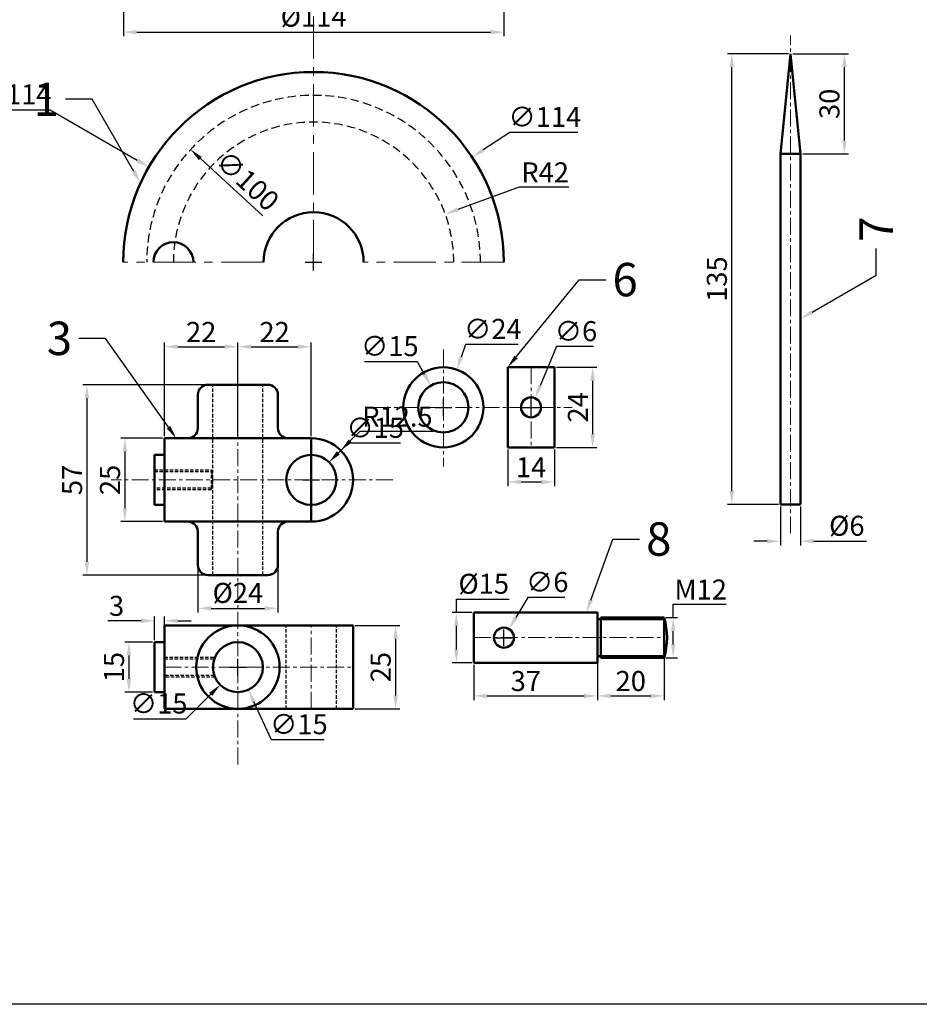
# Model space of a CAD drawing. Units: millimetres. Extents: x -65 to 576, y -103 to 374.
# Tile 2 of 4: x 81 to 351, y -103 to 192. Entities that reach past the tile are written whole.
import ezdxf
from ezdxf import colors
from ezdxf.entities.mleader import LeaderData, LeaderLine
from ezdxf.math import Vec2, Vec3

# ---------------------------------------------------------------- set-up
doc = ezdxf.new("R2010")
doc.units = ezdxf.units.MM
doc.header["$LTSCALE"] = 0.4
doc.linetypes.add('CENTER', pattern=[50.8, 31.75, -6.35, 6.35, -6.35])
doc.linetypes.add('HIDDEN', pattern=[9.525, 6.35, -3.175])
for name, color, linetype, lineweight in [('M-CNTR', 4, 'CENTER', 18), ('M-DIMS', 2, 'Continuous', 25), ('M-HIDN', 1, 'HIDDEN', 25), ('M-OUTL', 7, 'Continuous', 50), ('M-TEXT', 3, 'Continuous', 25), ('M-TTLB', 7, 'Continuous', 25)]:
    doc.layers.add(name, color=color, linetype=linetype, lineweight=lineweight)
doc.styles.get("Standard").update_dxf_attribs({"font": 'arial.ttf'})
doc.dimstyles.new('ISO-25', dxfattribs={"dimtxt": 6, "dimasz": 4, "dimexe": 1.25, "dimexo": 0.625, "dimtad": 1, "dimtoh": 1, "dimtxsty": 'Standard', "dimcen": 2.5, "dimadec": 0, "dimazin": 0, "dimtfac": 1, "dimtofl": 0, "dimtmove": 0, "dimatfit": 3, "dimfxl": 1, "dimarcsym": 0})

# ---------------------------------------------------------------- blocks, each defined once
blk = doc.blocks.new('*D1')
at = {"layer": 'Defpoints', "color": 0, "ltscale": 0.4, "transparency": 16777216}
for p in [(112.15, 220.83), (226.15, 220.83), (226.15, 187.9)]:
    blk.add_point(p, dxfattribs=at)
at = {"layer": 'M-DIMS', "color": 0, "lineweight": -2, "ltscale": 0.4, "transparency": 16777216}
for p, q in [((112.15, 220.2), (112.15, 186.65)), ((226.15, 220.2), (226.15, 186.65)), ((116.15, 187.9), (222.15, 187.9))]:
    blk.add_line(p, q, dxfattribs=at)
at = {"layer": 'M-DIMS', "color": 0, "ltscale": 0.4, "transparency": 16777216}
for points in [[(116.15, 188.57), (116.15, 187.24), (112.15, 187.9)], [(222.15, 188.57), (222.15, 187.24), (226.15, 187.9)]]:
    blk.add_solid(points, dxfattribs=at)
at = {"layer": 'M-DIMS', "color": 0, "ltscale": 0.4, "transparency": 16777216, "insert": (169.15, 191.76), "char_height": 6, "attachment_point": 5}
blk.add_mtext('%%C114', dxfattribs=at)
blk = doc.blocks.new('*D8')
at = {"layer": 'Defpoints', "color": 0, "ltscale": 0.4, "transparency": 16777216}
for p in [(216.68, 150.42), (121.61, 87.5)]:
    blk.add_point(p, dxfattribs=at)
at = {"layer": 'M-DIMS', "color": 0, "lineweight": -2, "ltscale": 0.4, "transparency": 16777216}
for p, q in [((227.95, 157.88), (220.01, 152.63)), ((248.33, 157.88), (227.95, 157.88)), ((169.15, 116.46), (169.15, 121.46)), ((166.65, 118.96), (171.65, 118.96))]:
    blk.add_line(p, q, dxfattribs=at)
at = {"layer": 'M-DIMS', "color": 0, "ltscale": 0.4, "transparency": 16777216}
blk.add_solid([(219.64, 153.18), (220.38, 152.07), (216.68, 150.42)], dxfattribs=at)
at = {"layer": 'M-DIMS', "color": 0, "ltscale": 0.4, "transparency": 16777216, "insert": (238.45, 161.73), "char_height": 6, "attachment_point": 5}
blk.add_mtext('∅114', dxfattribs=at)
blk = doc.blocks.new('*D9')
at = {"layer": 'Defpoints', "color": 0, "ltscale": 0.4, "transparency": 16777216}
for p in [(132.28, 152.73), (206.01, 85.18)]:
    blk.add_point(p, dxfattribs=at)
at = {"layer": 'M-DIMS', "color": 0, "lineweight": -2, "ltscale": 0.4, "transparency": 16777216}
blk.add_line((153.98, 132.85), (135.23, 150.03), dxfattribs=at)
at = {"layer": 'M-DIMS', "color": 0, "ltscale": 0.4, "transparency": 16777216}
blk.add_solid([(135.68, 150.52), (134.78, 149.54), (132.28, 152.73)], dxfattribs=at)
at = {"layer": 'M-DIMS', "color": 0, "ltscale": 0.4, "transparency": 16777216, "insert": (148.84, 142.79), "char_height": 6, "attachment_point": 5, "rotation": 317.5054}
blk.add_mtext('∅100', dxfattribs=at)
blk = doc.blocks.new('*D10')
at = {"layer": 'Defpoints', "color": 0, "ltscale": 0.4, "transparency": 16777216}
for p in [(208.59, 133.37), (169.15, 118.96)]:
    blk.add_point(p, dxfattribs=at)
at = {"layer": 'M-DIMS', "color": 0, "lineweight": -2, "ltscale": 0.4, "transparency": 16777216}
for p, q in [((230.77, 141.47), (212.35, 134.75)), ((245.67, 141.47), (230.77, 141.47)), ((169.15, 116.46), (169.15, 121.46)), ((166.65, 118.96), (171.65, 118.96))]:
    blk.add_line(p, q, dxfattribs=at)
at = {"layer": 'M-DIMS', "color": 0, "ltscale": 0.4, "transparency": 16777216}
blk.add_solid([(212.12, 135.37), (212.58, 134.12), (208.59, 133.37)], dxfattribs=at)
at = {"layer": 'M-DIMS', "color": 0, "ltscale": 0.4, "transparency": 16777216, "insert": (238.53, 145.11), "char_height": 6, "attachment_point": 5}
blk.add_mtext('R42', dxfattribs=at)
blk = doc.blocks.new('*D24')
at = {"layer": 'Defpoints', "color": 0, "ltscale": 0.4, "transparency": 16777216}
for p in [(312.08, 181.41), (328.19, 181.41), (315.08, 151.41)]:
    blk.add_point(p, dxfattribs=at)
at = {"layer": 'M-DIMS', "color": 0, "lineweight": -2, "ltscale": 0.4, "transparency": 16777216}
for p, q in [((312.71, 181.41), (329.44, 181.41)), ((328.19, 155.41), (328.19, 177.41)), ((315.71, 151.41), (329.44, 151.41))]:
    blk.add_line(p, q, dxfattribs=at)
at = {"layer": 'M-DIMS', "color": 0, "ltscale": 0.4, "transparency": 16777216}
for points in [[(327.53, 177.41), (328.86, 177.41), (328.19, 181.41)], [(327.53, 155.41), (328.86, 155.41), (328.19, 151.41)]]:
    blk.add_solid(points, dxfattribs=at)
at = {"layer": 'M-DIMS', "color": 0, "ltscale": 0.4, "transparency": 16777216, "insert": (324.5, 166.41), "char_height": 6, "attachment_point": 5, "rotation": 90}
blk.add_mtext('30', dxfattribs=at)
blk = doc.blocks.new('*D25')
at = {"layer": 'Defpoints', "color": 0, "ltscale": 0.4, "transparency": 16777216}
for p in [(294.46, 181.41), (312.08, 181.41), (309.08, 46.41)]:
    blk.add_point(p, dxfattribs=at)
at = {"layer": 'M-DIMS', "color": 0, "lineweight": -2, "ltscale": 0.4, "transparency": 16777216}
for p, q in [((311.46, 181.41), (293.21, 181.41)), ((294.46, 50.41), (294.46, 177.41)), ((308.46, 46.41), (293.21, 46.41))]:
    blk.add_line(p, q, dxfattribs=at)
at = {"layer": 'M-DIMS', "color": 0, "ltscale": 0.4, "transparency": 16777216}
for points in [[(293.79, 177.41), (295.13, 177.41), (294.46, 181.41)], [(293.79, 50.41), (295.13, 50.41), (294.46, 46.41)]]:
    blk.add_solid(points, dxfattribs=at)
at = {"layer": 'M-DIMS', "color": 0, "ltscale": 0.4, "transparency": 16777216, "insert": (290.77, 113.91), "char_height": 6, "attachment_point": 5, "rotation": 90}
blk.add_mtext('135', dxfattribs=at)
blk = doc.blocks.new('*D26')
at = {"layer": 'Defpoints', "color": 0, "ltscale": 0.4, "transparency": 16777216}
for p in [(309.08, 46.41), (315.08, 46.41), (315.08, 35.37)]:
    blk.add_point(p, dxfattribs=at)
at = {"layer": 'M-DIMS', "color": 0, "lineweight": -2, "ltscale": 0.4, "transparency": 16777216}
for p, q in [((309.08, 45.79), (309.08, 34.12)), ((315.08, 45.79), (315.08, 34.12)), ((305.08, 35.37), (301.08, 35.37)), ((319.08, 35.37), (334.79, 35.37))]:
    blk.add_line(p, q, dxfattribs=at)
at = {"layer": 'M-DIMS', "color": 0, "ltscale": 0.4, "transparency": 16777216}
for points in [[(305.08, 36.04), (305.08, 34.71), (309.08, 35.37)], [(319.08, 36.04), (319.08, 34.71), (315.08, 35.37)]]:
    blk.add_solid(points, dxfattribs=at)
at = {"layer": 'M-DIMS', "color": 0, "ltscale": 0.4, "transparency": 16777216, "insert": (328.93, 39.23), "char_height": 6, "attachment_point": 5}
blk.add_mtext('%%C6', dxfattribs=at)
blk = doc.blocks.new('*D27')
at = {"layer": 'Defpoints', "color": 0, "ltscale": 0.4, "transparency": 16777216}
for p in [(227.31, 63.48), (241.31, 63.48), (241.31, 53.14)]:
    blk.add_point(p, dxfattribs=at)
at = {"layer": 'M-DIMS', "color": 0, "lineweight": -2, "ltscale": 0.4, "transparency": 16777216}
for p, q in [((227.31, 62.86), (227.31, 51.89)), ((241.31, 62.86), (241.31, 51.89)), ((231.31, 53.14), (237.31, 53.14))]:
    blk.add_line(p, q, dxfattribs=at)
at = {"layer": 'M-DIMS', "color": 0, "ltscale": 0.4, "transparency": 16777216}
for points in [[(231.31, 53.81), (231.31, 52.48), (227.31, 53.14)], [(237.31, 53.81), (237.31, 52.48), (241.31, 53.14)]]:
    blk.add_solid(points, dxfattribs=at)
at = {"layer": 'M-DIMS', "color": 0, "ltscale": 0.4, "transparency": 16777216, "insert": (234.31, 56.78), "char_height": 6, "attachment_point": 5}
blk.add_mtext('14', dxfattribs=at)
blk = doc.blocks.new('*D28')
at = {"layer": 'Defpoints', "color": 0, "ltscale": 0.4, "transparency": 16777216}
for p in [(241.31, 87.48), (241.31, 63.48), (252.77, 63.48)]:
    blk.add_point(p, dxfattribs=at)
at = {"layer": 'M-DIMS', "color": 0, "lineweight": -2, "ltscale": 0.4, "transparency": 16777216}
for p, q in [((241.94, 87.48), (254.02, 87.48)), ((252.77, 83.48), (252.77, 67.48)), ((241.94, 63.48), (254.02, 63.48))]:
    blk.add_line(p, q, dxfattribs=at)
at = {"layer": 'M-DIMS', "color": 0, "ltscale": 0.4, "transparency": 16777216}
for points in [[(252.1, 83.48), (253.44, 83.48), (252.77, 87.48)], [(252.1, 67.48), (253.44, 67.48), (252.77, 63.48)]]:
    blk.add_solid(points, dxfattribs=at)
at = {"layer": 'M-DIMS', "color": 0, "ltscale": 0.4, "transparency": 16777216, "insert": (249.13, 75.48), "char_height": 6, "attachment_point": 5, "rotation": 90}
blk.add_mtext('24', dxfattribs=at)
blk = doc.blocks.new('*D29')
at = {"layer": 'Defpoints', "color": 0, "ltscale": 0.4, "transparency": 16777216}
for p in [(124.47, 66.24), (112.62, 41.24), (124.47, 41.24)]:
    blk.add_point(p, dxfattribs=at)
at = {"layer": 'M-DIMS', "color": 0, "lineweight": -2, "ltscale": 0.4, "transparency": 16777216}
for p, q in [((123.85, 66.24), (111.37, 66.24)), ((112.62, 62.24), (112.62, 45.24)), ((123.85, 41.24), (111.37, 41.24))]:
    blk.add_line(p, q, dxfattribs=at)
at = {"layer": 'M-DIMS', "color": 0, "ltscale": 0.4, "transparency": 16777216}
for points in [[(111.95, 62.24), (113.29, 62.24), (112.62, 66.24)], [(111.95, 45.24), (113.29, 45.24), (112.62, 41.24)]]:
    blk.add_solid(points, dxfattribs=at)
at = {"layer": 'M-DIMS', "color": 0, "ltscale": 0.4, "transparency": 16777216, "insert": (108.93, 53.74), "char_height": 6, "attachment_point": 5, "rotation": 90}
blk.add_mtext('25', dxfattribs=at)
blk = doc.blocks.new('*D30')
at = {"layer": 'Defpoints', "color": 0, "ltscale": 0.4, "transparency": 16777216}
for p in [(142.37, 82.24), (101.24, 25.24), (142.37, 25.24)]:
    blk.add_point(p, dxfattribs=at)
at = {"layer": 'M-DIMS', "color": 0, "lineweight": -2, "ltscale": 0.4, "transparency": 16777216}
for p, q in [((141.75, 82.24), (99.99, 82.24)), ((101.24, 78.24), (101.24, 29.24)), ((141.75, 25.24), (99.99, 25.24))]:
    blk.add_line(p, q, dxfattribs=at)
at = {"layer": 'M-DIMS', "color": 0, "ltscale": 0.4, "transparency": 16777216}
for points in [[(100.57, 78.24), (101.91, 78.24), (101.24, 82.24)], [(100.57, 29.24), (101.91, 29.24), (101.24, 25.24)]]:
    blk.add_solid(points, dxfattribs=at)
at = {"layer": 'M-DIMS', "color": 0, "ltscale": 0.4, "transparency": 16777216, "insert": (97.57, 53.74), "char_height": 6, "attachment_point": 5, "rotation": 90}
blk.add_mtext('57', dxfattribs=at)
blk = doc.blocks.new('*D31')
at = {"layer": 'Defpoints', "color": 0, "ltscale": 0.4, "transparency": 16777216}
for p in [(146.47, 93.65), (124.47, 66.24), (146.47, 66.24)]:
    blk.add_point(p, dxfattribs=at)
at = {"layer": 'M-DIMS', "color": 0, "lineweight": -2, "ltscale": 0.4, "transparency": 16777216}
for p, q in [((124.47, 66.87), (124.47, 94.9)), ((146.47, 66.87), (146.47, 94.9)), ((128.47, 93.65), (142.47, 93.65))]:
    blk.add_line(p, q, dxfattribs=at)
at = {"layer": 'M-DIMS', "color": 0, "ltscale": 0.4, "transparency": 16777216}
for points in [[(128.47, 94.32), (128.47, 92.99), (124.47, 93.65)], [(142.47, 94.32), (142.47, 92.99), (146.47, 93.65)]]:
    blk.add_solid(points, dxfattribs=at)
at = {"layer": 'M-DIMS', "color": 0, "ltscale": 0.4, "transparency": 16777216, "insert": (135.47, 97.29), "char_height": 6, "attachment_point": 5}
blk.add_mtext('22', dxfattribs=at)
blk = doc.blocks.new('*D32')
at = {"layer": 'Defpoints', "color": 0, "ltscale": 0.4, "transparency": 16777216}
for p in [(168.47, 93.65), (146.47, 66.24), (168.47, 66.24)]:
    blk.add_point(p, dxfattribs=at)
at = {"layer": 'M-DIMS', "color": 0, "lineweight": -2, "ltscale": 0.4, "transparency": 16777216}
for p, q in [((146.47, 66.87), (146.47, 94.9)), ((168.47, 66.87), (168.47, 94.9)), ((150.47, 93.65), (164.47, 93.65))]:
    blk.add_line(p, q, dxfattribs=at)
at = {"layer": 'M-DIMS', "color": 0, "ltscale": 0.4, "transparency": 16777216}
for points in [[(150.47, 94.32), (150.47, 92.99), (146.47, 93.65)], [(164.47, 94.32), (164.47, 92.99), (168.47, 93.65)]]:
    blk.add_solid(points, dxfattribs=at)
at = {"layer": 'M-DIMS', "color": 0, "ltscale": 0.4, "transparency": 16777216, "insert": (157.47, 97.29), "char_height": 6, "attachment_point": 5}
blk.add_mtext('22', dxfattribs=at)
blk = doc.blocks.new('*D33')
at = {"layer": 'Defpoints', "color": 0, "ltscale": 0.4, "transparency": 16777216}
for p in [(124.47, 11.55), (121.47, 5.16), (124.47, 5.16)]:
    blk.add_point(p, dxfattribs=at)
at = {"layer": 'M-DIMS', "color": 0, "lineweight": -2, "ltscale": 0.4, "transparency": 16777216}
for p, q in [((121.47, 5.78), (121.47, 12.8)), ((124.47, 5.78), (124.47, 12.8)), ((117.47, 11.55), (107.53, 11.55)), ((128.47, 11.55), (132.47, 11.55))]:
    blk.add_line(p, q, dxfattribs=at)
at = {"layer": 'M-DIMS', "color": 0, "ltscale": 0.4, "transparency": 16777216}
for points in [[(117.47, 12.21), (117.47, 10.88), (121.47, 11.55)], [(128.47, 12.21), (128.47, 10.88), (124.47, 11.55)]]:
    blk.add_solid(points, dxfattribs=at)
at = {"layer": 'M-DIMS', "color": 0, "ltscale": 0.4, "transparency": 16777216, "insert": (110.12, 15.24), "char_height": 6, "attachment_point": 5}
blk.add_mtext('3', dxfattribs=at)
blk = doc.blocks.new('*D34')
at = {"layer": 'Defpoints', "color": 0, "ltscale": 0.4, "transparency": 16777216}
for p in [(121.47, 5.16), (113.81, -9.84), (121.47, -9.84)]:
    blk.add_point(p, dxfattribs=at)
at = {"layer": 'M-DIMS', "color": 0, "lineweight": -2, "ltscale": 0.4, "transparency": 16777216}
for p, q in [((120.85, 5.16), (112.56, 5.16)), ((113.81, 1.16), (113.81, -5.84)), ((120.85, -9.84), (112.56, -9.84))]:
    blk.add_line(p, q, dxfattribs=at)
at = {"layer": 'M-DIMS', "color": 0, "ltscale": 0.4, "transparency": 16777216}
for points in [[(113.14, 1.16), (114.48, 1.16), (113.81, 5.16)], [(113.14, -5.84), (114.48, -5.84), (113.81, -9.84)]]:
    blk.add_solid(points, dxfattribs=at)
at = {"layer": 'M-DIMS', "color": 0, "ltscale": 0.4, "transparency": 16777216, "insert": (110.12, -2.34), "char_height": 6, "attachment_point": 5, "rotation": 90}
blk.add_mtext('15', dxfattribs=at)
blk = doc.blocks.new('*D35')
at = {"layer": 'Defpoints', "color": 0, "ltscale": 0.4, "transparency": 16777216}
for p in [(212.03, 86.8), (204.04, 64.17)]:
    blk.add_point(p, dxfattribs=at)
at = {"layer": 'M-DIMS', "color": 0, "lineweight": -2, "ltscale": 0.4, "transparency": 16777216}
for p, q in [((214.7, 94.34), (213.36, 90.57)), ((230.42, 94.34), (214.7, 94.34)), ((208.04, 72.98), (208.04, 77.98)), ((205.54, 75.48), (210.54, 75.48))]:
    blk.add_line(p, q, dxfattribs=at)
at = {"layer": 'M-DIMS', "color": 0, "ltscale": 0.4, "transparency": 16777216}
blk.add_solid([(212.74, 90.79), (213.99, 90.35), (212.03, 86.8)], dxfattribs=at)
at = {"layer": 'M-DIMS', "color": 0, "ltscale": 0.4, "transparency": 16777216, "insert": (222.87, 98.2), "char_height": 6, "attachment_point": 5}
blk.add_mtext('∅24', dxfattribs=at)
blk = doc.blocks.new('*D36')
at = {"layer": 'Defpoints', "color": 0, "ltscale": 0.4, "transparency": 16777216}
for p in [(204.31, 82), (211.76, 68.97)]:
    blk.add_point(p, dxfattribs=at)
at = {"layer": 'M-DIMS', "color": 0, "lineweight": -2, "ltscale": 0.4, "transparency": 16777216}
for p, q in [((184.41, 89.19), (200.2, 89.19)), ((200.2, 89.19), (202.33, 85.47)), ((208.04, 72.98), (208.04, 77.98)), ((205.54, 75.48), (210.54, 75.48))]:
    blk.add_line(p, q, dxfattribs=at)
at = {"layer": 'M-DIMS', "color": 0, "ltscale": 0.4, "transparency": 16777216}
blk.add_solid([(202.91, 85.8), (201.75, 85.14), (204.31, 82)], dxfattribs=at)
at = {"layer": 'M-DIMS', "color": 0, "ltscale": 0.4, "transparency": 16777216, "insert": (191.99, 93.05), "char_height": 6, "attachment_point": 5}
blk.add_mtext('∅15', dxfattribs=at)
blk = doc.blocks.new('*D37')
at = {"layer": 'Defpoints', "color": 0, "ltscale": 0.4, "transparency": 16777216}
for p in [(235.47, 78.25), (233.15, 72.72)]:
    blk.add_point(p, dxfattribs=at)
at = {"layer": 'M-DIMS', "color": 0, "lineweight": -2, "ltscale": 0.4, "transparency": 16777216}
for p, q in [((241.92, 93.68), (237.01, 81.94)), ((253, 93.68), (241.92, 93.68)), ((234.31, 72.98), (234.31, 77.98)), ((231.81, 75.48), (236.81, 75.48))]:
    blk.add_line(p, q, dxfattribs=at)
at = {"layer": 'M-DIMS', "color": 0, "ltscale": 0.4, "transparency": 16777216}
blk.add_solid([(236.4, 82.2), (237.63, 81.69), (235.47, 78.25)], dxfattribs=at)
at = {"layer": 'M-DIMS', "color": 0, "ltscale": 0.4, "transparency": 16777216, "insert": (247.78, 97.54), "char_height": 6, "attachment_point": 5}
blk.add_mtext('∅6', dxfattribs=at)
blk = doc.blocks.new('*D38')
at = {"layer": 'Defpoints', "color": 0, "ltscale": 0.4, "transparency": 16777216}
for p in [(180.97, 10.16), (180.97, -14.84), (193.72, -14.84)]:
    blk.add_point(p, dxfattribs=at)
at = {"layer": 'M-DIMS', "color": 0, "lineweight": -2, "ltscale": 0.4, "transparency": 16777216}
for p, q in [((181.6, 10.16), (194.97, 10.16)), ((193.72, 6.16), (193.72, -10.84)), ((181.6, -14.84), (194.97, -14.84))]:
    blk.add_line(p, q, dxfattribs=at)
at = {"layer": 'M-DIMS', "color": 0, "ltscale": 0.4, "transparency": 16777216}
for points in [[(193.06, 6.16), (194.39, 6.16), (193.72, 10.16)], [(193.06, -10.84), (194.39, -10.84), (193.72, -14.84)]]:
    blk.add_solid(points, dxfattribs=at)
at = {"layer": 'M-DIMS', "color": 0, "ltscale": 0.4, "transparency": 16777216, "insert": (190.04, -2.34), "char_height": 6, "attachment_point": 5, "rotation": 90}
blk.add_mtext('25', dxfattribs=at)
blk = doc.blocks.new('*D39')
at = {"layer": 'Defpoints', "color": 0, "ltscale": 0.4, "transparency": 16777216}
for p in [(143.32, 4.46), (149.62, -9.15)]:
    blk.add_point(p, dxfattribs=at)
at = {"layer": 'M-DIMS', "color": 0, "lineweight": -2, "ltscale": 0.4, "transparency": 16777216}
for p, q in [((146.47, -4.84), (146.47, 0.16)), ((143.97, -2.34), (148.97, -2.34)), ((156.54, -24.09), (151.3, -12.78)), ((172.33, -24.09), (156.54, -24.09))]:
    blk.add_line(p, q, dxfattribs=at)
at = {"layer": 'M-DIMS', "color": 0, "ltscale": 0.4, "transparency": 16777216}
blk.add_solid([(151.91, -12.5), (150.7, -13.06), (149.62, -9.15)], dxfattribs=at)
at = {"layer": 'M-DIMS', "color": 0, "ltscale": 0.4, "transparency": 16777216, "insert": (164.75, -20.24), "char_height": 6, "attachment_point": 5}
blk.add_mtext('∅15', dxfattribs=at)
blk = doc.blocks.new('*D40')
at = {"layer": 'Defpoints', "color": 0, "ltscale": 0.4, "transparency": 16777216}
for p in [(134.47, 33.24), (158.47, 33.24), (158.47, 15.27)]:
    blk.add_point(p, dxfattribs=at)
at = {"layer": 'M-DIMS', "color": 0, "lineweight": -2, "ltscale": 0.4, "transparency": 16777216}
for p, q in [((134.47, 32.62), (134.47, 14.02)), ((158.47, 32.62), (158.47, 14.02)), ((138.47, 15.27), (154.47, 15.27))]:
    blk.add_line(p, q, dxfattribs=at)
at = {"layer": 'M-DIMS', "color": 0, "ltscale": 0.4, "transparency": 16777216}
for points in [[(138.47, 15.93), (138.47, 14.6), (134.47, 15.27)], [(154.47, 15.93), (154.47, 14.6), (158.47, 15.27)]]:
    blk.add_solid(points, dxfattribs=at)
at = {"layer": 'M-DIMS', "color": 0, "ltscale": 0.4, "transparency": 16777216, "insert": (146.47, 19.12), "char_height": 6, "attachment_point": 5}
blk.add_mtext('%%C24', dxfattribs=at)
blk = doc.blocks.new('*D41')
at = {"layer": 'Defpoints', "color": 0, "ltscale": 0.4, "transparency": 16777216}
for p in [(217.19, 13.98), (211.93, -1.02), (217.19, -1.02)]:
    blk.add_point(p, dxfattribs=at)
at = {"layer": 'M-DIMS', "color": 0, "lineweight": -2, "ltscale": 0.4, "transparency": 16777216}
for p, q in [((211.93, 13.98), (211.93, 17.98)), ((211.93, 17.98), (227.72, 17.98)), ((216.57, 13.98), (210.68, 13.98)), ((211.93, 2.98), (211.93, 9.98)), ((216.57, -1.02), (210.68, -1.02))]:
    blk.add_line(p, q, dxfattribs=at)
at = {"layer": 'M-DIMS', "color": 0, "ltscale": 0.4, "transparency": 16777216}
for points in [[(211.27, 9.98), (212.6, 9.98), (211.93, 13.98)], [(211.27, 2.98), (212.6, 2.98), (211.93, -1.02)]]:
    blk.add_solid(points, dxfattribs=at)
at = {"layer": 'M-DIMS', "color": 0, "ltscale": 0.4, "transparency": 16777216, "insert": (220.14, 21.84), "char_height": 6, "attachment_point": 5}
blk.add_mtext('%%C15', dxfattribs=at)
blk = doc.blocks.new('*D42')
at = {"layer": 'Defpoints', "color": 0, "ltscale": 0.4, "transparency": 16777216}
for p in [(227.72, 9.07), (224.67, 3.9)]:
    blk.add_point(p, dxfattribs=at)
at = {"layer": 'M-DIMS', "color": 0, "lineweight": -2, "ltscale": 0.4, "transparency": 16777216}
for p, q in [((233.31, 18.54), (229.75, 12.51)), ((244.39, 18.54), (233.31, 18.54)), ((226.19, 3.98), (226.19, 8.98)), ((223.69, 6.48), (228.69, 6.48))]:
    blk.add_line(p, q, dxfattribs=at)
at = {"layer": 'M-DIMS', "color": 0, "ltscale": 0.4, "transparency": 16777216}
blk.add_solid([(229.18, 12.85), (230.33, 12.17), (227.72, 9.07)], dxfattribs=at)
at = {"layer": 'M-DIMS', "color": 0, "ltscale": 0.4, "transparency": 16777216, "insert": (239.16, 22.39), "char_height": 6, "attachment_point": 5}
blk.add_mtext('∅6', dxfattribs=at)
blk = doc.blocks.new('*D43')
at = {"layer": 'Defpoints', "color": 0, "ltscale": 0.4, "transparency": 16777216}
for p in [(217.19, -1.02), (254.19, -1.02), (254.19, -10.97)]:
    blk.add_point(p, dxfattribs=at)
at = {"layer": 'M-DIMS', "color": 0, "lineweight": -2, "ltscale": 0.4, "transparency": 16777216}
for p, q in [((217.19, -1.64), (217.19, -12.22)), ((254.19, -1.64), (254.19, -12.22)), ((221.19, -10.97), (250.19, -10.97))]:
    blk.add_line(p, q, dxfattribs=at)
at = {"layer": 'M-DIMS', "color": 0, "ltscale": 0.4, "transparency": 16777216}
for points in [[(221.19, -10.31), (221.19, -11.64), (217.19, -10.97)], [(250.19, -10.31), (250.19, -11.64), (254.19, -10.97)]]:
    blk.add_solid(points, dxfattribs=at)
at = {"layer": 'M-DIMS', "color": 0, "ltscale": 0.4, "transparency": 16777216, "insert": (232.75, -7.28), "char_height": 6, "attachment_point": 5}
blk.add_mtext('37', dxfattribs=at)
blk = doc.blocks.new('*D44')
at = {"layer": 'Defpoints', "color": 0, "ltscale": 0.4, "transparency": 16777216}
for p in [(254.19, 6.48), (274.19, 6.48), (274.19, -10.97)]:
    blk.add_point(p, dxfattribs=at)
at = {"layer": 'M-DIMS', "color": 0, "lineweight": -2, "ltscale": 0.4, "transparency": 16777216}
for p, q in [((254.19, 5.86), (254.19, -12.22)), ((274.19, 5.86), (274.19, -12.22)), ((258.19, -10.97), (270.19, -10.97))]:
    blk.add_line(p, q, dxfattribs=at)
at = {"layer": 'M-DIMS', "color": 0, "ltscale": 0.4, "transparency": 16777216}
for points in [[(258.19, -10.31), (258.19, -11.64), (254.19, -10.97)], [(270.19, -10.31), (270.19, -11.64), (274.19, -10.97)]]:
    blk.add_solid(points, dxfattribs=at)
at = {"layer": 'M-DIMS', "color": 0, "ltscale": 0.4, "transparency": 16777216, "insert": (264.19, -7.28), "char_height": 6, "attachment_point": 5}
blk.add_mtext('20', dxfattribs=at)
blk = doc.blocks.new('*D45')
at = {"layer": 'Defpoints', "color": 0, "ltscale": 0.4, "transparency": 16777216}
for p in [(274.19, 12.48), (274.19, 0.48), (276.9, 0.48)]:
    blk.add_point(p, dxfattribs=at)
at = {"layer": 'M-DIMS', "color": 0, "lineweight": -2, "ltscale": 0.4, "transparency": 16777216}
for p, q in [((276.9, 12.48), (276.9, 16.48)), ((276.9, 16.48), (292.76, 16.48)), ((274.82, 12.48), (278.15, 12.48)), ((276.9, 4.48), (276.9, 8.48)), ((274.82, 0.48), (278.15, 0.48))]:
    blk.add_line(p, q, dxfattribs=at)
at = {"layer": 'M-DIMS', "color": 0, "ltscale": 0.4, "transparency": 16777216}
for points in [[(276.23, 8.48), (277.56, 8.48), (276.9, 12.48)], [(276.23, 4.48), (277.56, 4.48), (276.9, 0.48)]]:
    blk.add_solid(points, dxfattribs=at)
at = {"layer": 'M-DIMS', "color": 0, "ltscale": 0.4, "transparency": 16777216, "insert": (285.14, 20.12), "char_height": 6, "attachment_point": 5}
blk.add_mtext('M12', dxfattribs=at)
blk = doc.blocks.new('*D56')
at = {"layer": 'Defpoints', "color": 0, "ltscale": 0.4, "transparency": 16777216}
for p in [(119.8, 147.5), (218.49, 90.42)]:
    blk.add_point(p, dxfattribs=at)
at = {"layer": 'M-DIMS', "color": 0, "lineweight": -2, "ltscale": 0.4, "transparency": 16777216}
for p, q in [((69.82, 164.62), (90.2, 164.62)), ((90.2, 164.62), (116.34, 149.5)), ((169.15, 116.46), (169.15, 121.46)), ((166.65, 118.96), (171.65, 118.96))]:
    blk.add_line(p, q, dxfattribs=at)
at = {"layer": 'M-DIMS', "color": 0, "ltscale": 0.4, "transparency": 16777216}
blk.add_solid([(116.68, 150.08), (116.01, 148.92), (119.8, 147.5)], dxfattribs=at)
at = {"layer": 'M-DIMS', "color": 0, "ltscale": 0.4, "transparency": 16777216, "insert": (79.7, 168.48), "char_height": 6, "attachment_point": 5}
blk.add_mtext('∅114', dxfattribs=at)
blk = doc.blocks.new('*D57')
at = {"layer": 'Defpoints', "color": 0, "ltscale": 0.4, "transparency": 16777216}
for p in [(173.77, 59.05), (163.17, 48.44)]:
    blk.add_point(p, dxfattribs=at)
at = {"layer": 'M-DIMS', "color": 0, "lineweight": -2, "ltscale": 0.4, "transparency": 16777216}
for p, q in [((179.42, 64.71), (176.6, 61.88)), ((195.22, 64.71), (179.42, 64.71)), ((168.47, 51.24), (168.47, 56.24)), ((165.97, 53.74), (170.97, 53.74))]:
    blk.add_line(p, q, dxfattribs=at)
at = {"layer": 'M-DIMS', "color": 0, "ltscale": 0.4, "transparency": 16777216}
blk.add_solid([(176.13, 62.35), (177.07, 61.41), (173.77, 59.05)], dxfattribs=at)
at = {"layer": 'M-DIMS', "color": 0, "ltscale": 0.4, "transparency": 16777216, "insert": (187.63, 68.57), "char_height": 6, "attachment_point": 5}
blk.add_mtext('∅15', dxfattribs=at)
blk = doc.blocks.new('*D58')
at = {"layer": 'Defpoints', "color": 0, "ltscale": 0.4, "transparency": 16777216}
for p in [(177.31, 62.58), (168.47, 53.74)]:
    blk.add_point(p, dxfattribs=at)
at = {"layer": 'M-DIMS', "color": 0, "lineweight": -2, "ltscale": 0.4, "transparency": 16777216}
for p, q in [((182.97, 68.24), (180.14, 65.41)), ((204.97, 68.24), (182.97, 68.24)), ((168.47, 51.24), (168.47, 56.24)), ((165.97, 53.74), (170.97, 53.74))]:
    blk.add_line(p, q, dxfattribs=at)
at = {"layer": 'M-DIMS', "color": 0, "ltscale": 0.4, "transparency": 16777216}
blk.add_solid([(179.67, 65.88), (180.61, 64.94), (177.31, 62.58)], dxfattribs=at)
at = {"layer": 'M-DIMS', "color": 0, "ltscale": 0.4, "transparency": 16777216, "insert": (194.28, 71.93), "char_height": 6, "attachment_point": 5}
blk.add_mtext('R12.5', dxfattribs=at)
blk = doc.blocks.new('*D59')
at = {"layer": 'Defpoints', "color": 0, "ltscale": 0.4, "transparency": 16777216}
for p in [(151.77, 2.96), (141.17, -7.65)]:
    blk.add_point(p, dxfattribs=at)
at = {"layer": 'M-DIMS', "color": 0, "lineweight": -2, "ltscale": 0.4, "transparency": 16777216}
for p, q in [((146.47, -4.84), (146.47, 0.16)), ((143.97, -2.34), (148.97, -2.34)), ((130.95, -17.88), (138.34, -10.48)), ((115.15, -17.88), (130.95, -17.88))]:
    blk.add_line(p, q, dxfattribs=at)
at = {"layer": 'M-DIMS', "color": 0, "ltscale": 0.4, "transparency": 16777216}
blk.add_solid([(137.87, -10.01), (138.81, -10.95), (141.17, -7.65)], dxfattribs=at)
at = {"layer": 'M-DIMS', "color": 0, "ltscale": 0.4, "transparency": 16777216, "insert": (122.74, -14.02), "char_height": 6, "attachment_point": 5}
blk.add_mtext('∅15', dxfattribs=at)

msp = doc.modelspace()

# ---------------------------------------------------------------- linework, layer by layer
at = {"layer": 'M-CNTR'}
for p, q in [((169.146, 118.958), (169.146, 248.195)), ((154.146, 118.958), (112.146, 118.958)), ((226.146, 118.958), (184.146, 118.958))]:
    msp.add_line(p, q, dxfattribs=at)
at = {"layer": 'M-CNTR', "ltscale": 0.4}
for p, q in [((312.081, 37.744), (312.081, 186.935)), ((208.038, 92.848), (208.038, 57.733)), ((234.311, 87.485), (234.311, 63.485)), ((146.472, -31.53), (146.472, 82.245)), ((187.247, 75.485), (246.603, 75.485)), ((192.89, 53.745), (108.531, 53.745)), ((168.472, -14.845), (168.472, 10.155)), ((217.192, 6.484), (274.192, 6.484)), ((124.472, -2.345), (180.972, -2.345))]:
    msp.add_line(p, q, dxfattribs=at)
at = {"layer": 'M-HIDN', "ltscale": 0.4}
for p, q in [((138.972, 25.245), (138.972, 82.245)), ((153.972, 25.245), (153.972, 82.245)), ((121.472, 56.745), (138.472, 56.745)), ((121.472, 56.245), (138.472, 56.245)), ((138.472, 56.745), (138.472, 50.745)), ((138.472, 51.245), (121.472, 51.245)), ((138.472, 50.745), (121.472, 50.745)), ((160.972, -14.845), (160.972, 10.155)), ((175.972, -14.845), (175.972, 10.155)), ((124.472, 0.655), (139.598, 0.655)), ((124.472, 0.155), (139.401, 0.155)), ((139.401, -4.845), (124.472, -4.845)), ((139.598, -5.345), (124.472, -5.345))]:
    msp.add_line(p, q, dxfattribs=at)
at = {"layer": 'M-HIDN'}
for radius in [50, 42]:
    msp.add_arc((169.146, 118.958), radius, 0, 180, dxfattribs=at)
at = {"layer": 'M-HIDN', "ltscale": 0.4}
msp.add_arc((128.842, 53.745), 10.086, 342.69568, 17.30432, dxfattribs=at)
at = {"layer": 'M-OUTL', "ltscale": 0.4}
for p, q in [((309.081, 151.411), (312.081, 181.411)), ((312.081, 181.411), (315.081, 151.411)), ((309.081, 46.411), (309.081, 151.411)), ((309.081, 151.411), (315.081, 151.411)), ((315.081, 151.411), (315.081, 46.411)), ((227.311, 87.485), (227.311, 63.485)), ((241.311, 87.485), (227.311, 87.485)), ((241.311, 63.485), (241.311, 87.485)), ((155.472, 82.245), (137.472, 82.245)), ((134.472, 69.245), (134.472, 79.245)), ((158.472, 69.245), (158.472, 79.245)), ((124.472, 41.245), (124.472, 66.245)), ((124.472, 66.245), (131.472, 66.245)), ((131.472, 66.245), (161.472, 66.245)), ((161.472, 66.245), (168.472, 66.245)), ((168.472, 41.245), (168.472, 66.245)), ((227.311, 63.485), (241.311, 63.485)), ((124.472, 61.245), (121.472, 61.245)), ((121.472, 61.245), (121.472, 46.245)), ((121.472, 46.245), (124.472, 46.245)), ((315.081, 46.411), (309.081, 46.411)), ((131.472, 41.245), (124.472, 41.245)), ((161.472, 41.245), (131.472, 41.245)), ((168.472, 41.245), (161.472, 41.245)), ((134.472, 28.245), (134.472, 38.245)), ((158.472, 28.245), (158.472, 38.245)), ((155.472, 25.245), (137.472, 25.245)), ((217.192, 13.984), (217.192, -1.016)), ((254.192, 13.984), (217.192, 13.984)), ((254.192, -1.016), (254.192, 13.984)), ((254.192, 11.984), (274.192, 11.984)), ((255.192, 12.484), (274.192, 12.484)), ((255.192, 0.484), (255.192, 12.484)), ((274.192, 12.484), (274.192, 0.484)), ((124.472, -14.845), (124.472, 10.155)), ((124.472, 10.155), (131.472, 10.155)), ((131.472, 10.155), (180.972, 10.155)), ((161.472, 10.155), (168.472, 10.155)), ((180.972, -14.845), (180.972, 10.155)), ((124.472, 5.155), (121.472, 5.155)), ((121.472, 5.155), (121.472, -9.845)), ((274.192, 0.984), (254.192, 0.984)), ((274.192, 0.484), (255.192, 0.484)), ((217.192, -1.016), (254.192, -1.016)), ((121.472, -9.845), (124.472, -9.845)), ((131.472, -14.845), (124.472, -14.845)), ((180.972, -14.845), (131.472, -14.845)), ((168.472, -14.845), (161.472, -14.845))]:
    msp.add_line(p, q, dxfattribs=at)
for centre, radius in [((208.038, 75.485), 12), ((208.038, 75.485), 7.5), ((234.311, 75.485), 3), ((168.472, 53.745), 7.5), ((146.472, -2.345), 12.5), ((226.192, 6.484), 3), ((146.472, -2.345), 7.5)]:
    msp.add_circle(centre, radius, dxfattribs=at)
at = {"layer": 'M-OUTL'}
for radius in [57, 15]:
    msp.add_arc((169.146, 118.958), radius, 0, 180, dxfattribs=at)
at = {"layer": 'M-OUTL', "ltscale": 0.4}
for centre, radius, start, end in [((127.146, 118.958), 6, 0, 180), ((137.472, 79.245), 3, 90, 180), ((155.472, 79.245), 3, 0, 90), ((131.472, 69.245), 3, 270, 0), ((161.472, 69.245), 3, 180, 270), ((168.472, 53.745), 12.5, 270, 90), ((131.472, 38.245), 3, 0, 90), ((161.472, 38.245), 3, 90, 180), ((137.472, 28.245), 3, 180, 270), ((155.472, 28.245), 3, 270, 0), ((253.736, 6.484), 21.318, 343.65297, 16.34703)]:
    msp.add_arc(centre, radius, start, end, dxfattribs=at)
at = {"layer": 'M-TTLB', "ltscale": 0.4}
msp.add_lwpolyline([(-64.629, 373.834), (576.345, 373.834), (576.345, -103.363), (-64.629, -103.363)], close=True, dxfattribs=at)

# ---------------------------------------------------------------- dimensions: what is measured, and where the dimension line sits
at = {"layer": 'M-DIMS', "ltscale": 0.4}
dim = msp.add_linear_dim(base=(226.146, 187.903), p1=(112.146, 220.828), p2=(226.146, 220.828), text='%%C<>', dimstyle='ISO-25', override={"dimclrd": 0, "dimclre": 0, "dimclrt": 0}, dxfattribs=at)
dim.commit()
dim.dimension.update_dxf_attribs({"geometry": '*D1', "text_midpoint": (169.146, 187.903), "dimtype": 160})
for base, p1, p2, picture, middle in [((294.459, 181.411), (309.081, 46.411), (312.081, 181.411), '*D25', (290.768, 113.911)), ((328.192, 181.411), (315.081, 151.411), (312.081, 181.411), '*D24', (324.502, 166.411)), ((252.769, 63.485), (241.311, 87.485), (241.311, 63.485), '*D28', (249.132, 75.485)), ((101.241, 25.245), (142.374, 82.245), (142.374, 25.245), '*D30', (97.565, 53.745)), ((112.621, 41.245), (124.472, 66.245), (124.472, 41.245), '*D29', (108.933, 53.745)), ((193.723, -14.845), (180.972, 10.155), (180.972, -14.845), '*D38', (190.035, -2.345)), ((113.81, -9.845), (121.472, 5.155), (121.472, -9.845), '*D34', (110.121, -2.345))]:
    dim = msp.add_linear_dim(base=base, p1=p1, p2=p2, angle=90, dimstyle='ISO-25', override={"dimclrd": 0, "dimclre": 0, "dimclrt": 0}, dxfattribs=at)
    dim.commit()
    dim.dimension.update_dxf_attribs({"geometry": picture, "text_midpoint": middle})
for p1, p2, override, picture, middle in [((218.486, 90.418), (119.805, 147.497), {"dimdec": 0, "dimlfac": 1, "dimrnd": 0, "dimzin": 0, "dimdsep": 46, "dimlunit": 2}, '*D56', (79.696, 164.621)), ((121.614, 87.497), (216.677, 150.418), {"dimclrd": 0, "dimclre": 0, "dimclrt": 0}, '*D8', (238.453, 157.878)), ((206.013, 85.182), (132.279, 152.734), {"dimclrd": 0, "dimclre": 0, "dimclrt": 0}, '*D9', (146.233, 139.949)), ((233.154, 72.717), (235.468, 78.252), {"dimclrd": 0, "dimclre": 0, "dimclrt": 0}, '*D37', (247.775, 93.685)), ((211.761, 68.974), (204.314, 81.995), {"dimclrd": 0, "dimclre": 0, "dimclrt": 0}, '*D36', (191.99, 89.192)), ((163.172, 48.438), (173.771, 59.051), {"dimdec": 0, "dimlfac": 1, "dimrnd": 0, "dimzin": 0, "dimdsep": 46, "dimlunit": 2}, '*D57', (187.633, 64.712)), ((224.667, 3.901), (227.718, 9.067), {"dimclrd": 0, "dimclre": 0, "dimclrt": 0}, '*D42', (239.165, 18.535)), ((151.773, 2.96), (141.17, -7.65), {"dimdec": 0, "dimlfac": 1, "dimrnd": 0, "dimzin": 0, "dimdsep": 46, "dimlunit": 2}, '*D59', (122.738, -17.88)), ((143.32, 4.461), (149.623, -9.151), {"dimclrd": 0, "dimclre": 0, "dimclrt": 0}, '*D39', (164.751, -24.094))]:
    dim = msp.add_diameter_dim_2p(p1=p1, p2=p2, dimstyle='ISO-25', override=override, dxfattribs=at)
    dim.commit()
    dim.dimension.update_dxf_attribs({"geometry": picture, "text_midpoint": middle, "dimtype": 163})
dim = msp.add_radius_dim(center=(169.146, 118.958), mpoint=(208.594, 133.373), dimstyle='ISO-25', override={"dimclrd": 0, "dimclre": 0, "dimclrt": 0}, dxfattribs=at)
dim.commit()
dim.dimension.update_dxf_attribs({"geometry": '*D10', "text_midpoint": (238.528, 141.474), "dimtype": 164})
for base, p1, p2, picture, middle in [((146.472, 93.653), (124.472, 66.245), (146.472, 66.245), '*D31', (135.472, 97.29)), ((168.472, 93.653), (146.472, 66.245), (168.472, 66.245), '*D32', (157.472, 97.29)), ((241.311, 53.142), (227.311, 63.485), (241.311, 63.485), '*D27', (234.311, 56.779)), ((274.192, -10.972), (254.192, 6.484), (274.192, 6.484), '*D44', (264.192, -7.284))]:
    dim = msp.add_linear_dim(base=base, p1=p1, p2=p2, dimstyle='ISO-25', override={"dimclrd": 0, "dimclre": 0, "dimclrt": 0}, dxfattribs=at)
    dim.commit()
    dim.dimension.update_dxf_attribs({"geometry": picture, "text_midpoint": middle})
dim = msp.add_diameter_dim_2p(p1=(204.043, 64.169), p2=(212.033, 86.8), dimstyle='ISO-25', override={"dimclrd": 0, "dimclre": 0, "dimclrt": 0}, dxfattribs=at)
dim.commit()
dim.dimension.update_dxf_attribs({"geometry": '*D35', "text_midpoint": (222.87, 98.2)})
dim = msp.add_radius_dim(center=(168.472, 53.745), mpoint=(177.312, 62.582), dimstyle='ISO-25', override={"dimdec": 1, "dimlfac": 1, "dimrnd": 0, "dimzin": 0, "dimdsep": 46, "dimlunit": 2}, dxfattribs=at)
dim.commit()
dim.dimension.update_dxf_attribs({"geometry": '*D58', "text_midpoint": (194.281, 71.926)})
dim = msp.add_linear_dim(base=(315.081, 35.373), p1=(309.081, 46.411), p2=(315.081, 46.411), angle=180, text='%%C<>', dimstyle='ISO-25', override={"dimclrd": 0, "dimclre": 0, "dimclrt": 0}, dxfattribs=at)
dim.commit()
dim.dimension.update_dxf_attribs({"geometry": '*D26', "text_midpoint": (328.934, 39.23)})
dim = msp.add_linear_dim(base=(158.472, 15.268), p1=(134.472, 33.245), p2=(158.472, 33.245), text='%%C<>', dimstyle='ISO-25', override={"dimclrd": 0, "dimclre": 0, "dimclrt": 0}, dxfattribs=at)
dim.commit()
dim.dimension.update_dxf_attribs({"geometry": '*D40', "text_midpoint": (146.472, 19.124)})
for base, p1, p2, text, picture, middle in [((211.932, -1.016), (217.192, 13.984), (217.192, -1.016), '%%C<>', '*D41', (220.141, 17.984)), ((276.897, 0.484), (274.192, 12.484), (274.192, 0.484), 'M<>', '*D45', (285.143, 16.484))]:
    dim = msp.add_linear_dim(base=base, p1=p1, p2=p2, angle=90, text=text, dimstyle='ISO-25', override={"dimclrd": 0, "dimclre": 0, "dimclrt": 0}, dxfattribs=at)
    dim.commit()
    dim.dimension.update_dxf_attribs({"geometry": picture, "text_midpoint": middle, "dimtype": 160})
for base, p1, p2, picture, middle in [((124.472, 11.546), (121.472, 5.155), (124.472, 5.155), '*D33', (110.123, 11.546)), ((254.192, -10.972), (217.192, -1.016), (254.192, -1.016), '*D43', (232.747, -10.972))]:
    dim = msp.add_linear_dim(base=base, p1=p1, p2=p2, dimstyle='ISO-25', override={"dimclrd": 0, "dimclre": 0, "dimclrt": 0}, dxfattribs=at)
    dim.commit()
    dim.dimension.update_dxf_attribs({"geometry": picture, "text_midpoint": middle, "dimtype": 160})

# ---------------------------------------------------------------- leaders
at = {"layer": 'M-TEXT', "ltscale": 0.4}
ml = msp.add_multileader_mtext('Standard', dxfattribs=at)
ml.set_content('1', color=256)
ml.set_leader_properties()
ml.build(insert=Vec2(0, 0))
ctx = ml.context
ctx.base_point, ctx.char_height, ctx.plane_origin = Vec3(87.133, 167.794), 10, Vec3(117.316, 142.679)
ctx.text_align_type = 2
notes = []
notes.append((ctx, [(0, (1, 1, 0), (102.816, 167.794), (-1, 0), 8, [(0, [(117.316, 142.679)], 0, [])])]))
ctx.mtext.insert, ctx.mtext.alignment, ctx.mtext.flow_direction = Vec3(92.816, 172.794), 3, 5
ml = msp.add_multileader_mtext('Standard', dxfattribs=at)
ml.set_content('7', color=256)
ml.set_leader_properties()
ml.build(insert=Vec2(0, 0))
ctx = ml.context
ctx.base_point, ctx.char_height, ctx.plane_origin, ctx.plane_x_axis, ctx.plane_y_axis = Vec3(337.727, 123.094), 10, Vec3(315.081, 102.019), Vec3(0, 1), Vec3(-1, 0)
notes.append((ctx, [(0, (1, 1, 0), (337.727, 115.094), (0, 1), 8, [(0, [(315.081, 102.019)], 0, [])])]))
ctx.mtext.insert, ctx.mtext.text_direction, ctx.mtext.rotation, ctx.mtext.flow_direction = Vec3(332.727, 125.094), Vec3(0, 1), 1.5707963, 5
ml = msp.add_multileader_mtext('Standard', dxfattribs=at)
ml.set_content('6', color=256)
ml.set_leader_properties()
ml.build(insert=Vec2(0, 0))
ctx = ml.context
ctx.base_point, ctx.char_height, ctx.plane_origin = Vec3(256.712, 113.672), 10, Vec3(227.311, 87.485)
notes.append((ctx, [(0, (1, 1, 0), (248.712, 113.672), (1, 0), 8, [(0, [(227.311, 87.485)], 0, [])])]))
ctx.mtext.insert, ctx.mtext.flow_direction = Vec3(258.712, 118.757), 5
ml = msp.add_multileader_mtext('Standard', dxfattribs=at)
ml.set_content('3', color=256)
ml.set_leader_properties()
ml.build(insert=Vec2(0, 0))
ctx = ml.context
ctx.base_point, ctx.char_height, ctx.plane_origin = Vec3(88.231, 96.074), 10, Vec3(127.972, 66.245)
ctx.text_align_type = 2
notes.append((ctx, [(0, (1, 1, 0), (106.779, 96.074), (-1, 0), 8, [(0, [(127.972, 66.245)], 0, [])])]))
ctx.mtext.insert, ctx.mtext.alignment, ctx.mtext.flow_direction = Vec3(96.779, 101.163), 3, 5
ml = msp.add_multileader_mtext('Standard', dxfattribs=at)
ml.set_content('8', color=256)
ml.set_leader_properties()
ml.build(insert=Vec2(0, 0))
ctx = ml.context
ctx.base_point, ctx.char_height, ctx.plane_origin = Vec3(266.8, 35.955), 10, Vec3(250.86, 13.984)
notes.append((ctx, [(0, (1, 1, 0), (258.8, 35.955), (1, 0), 8, [(0, [(250.86, 13.984)], 0, [])])]))
ctx.mtext.insert, ctx.mtext.flow_direction = Vec3(268.8, 41.04), 5
for ctx, leaders in notes:
    for number, flags, end, landing, length, lines in leaders:
        leader = LeaderData()
        leader.index, (leader.has_last_leader_line, leader.has_dogleg_vector, leader.attachment_direction) = number, flags
        leader.last_leader_point, leader.dogleg_vector, leader.dogleg_length = Vec3(end), Vec3(landing), length
        for number, points, colour, breaks in lines:
            line = LeaderLine()
            line.index, line.vertices, line.color, line.breaks = number, Vec3.list(points), colors.encode_raw_color(colour), breaks
            leader.lines.append(line)
        ctx.leaders.append(leader)

doc.saveas('drawing.dxf')
